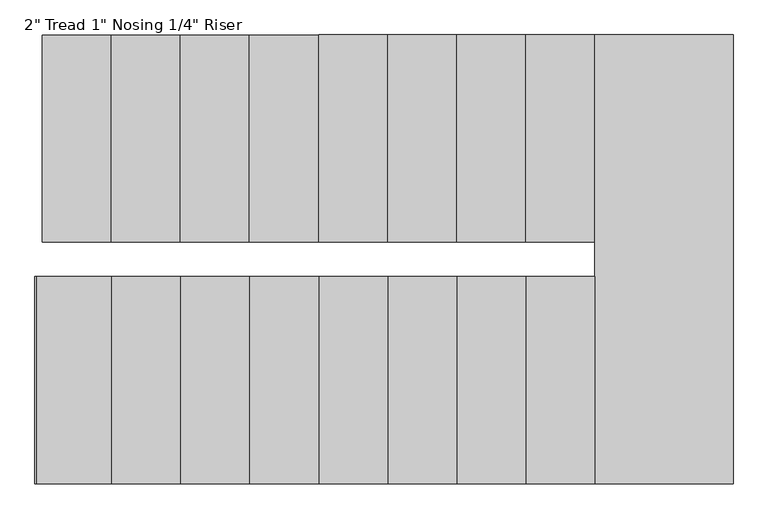
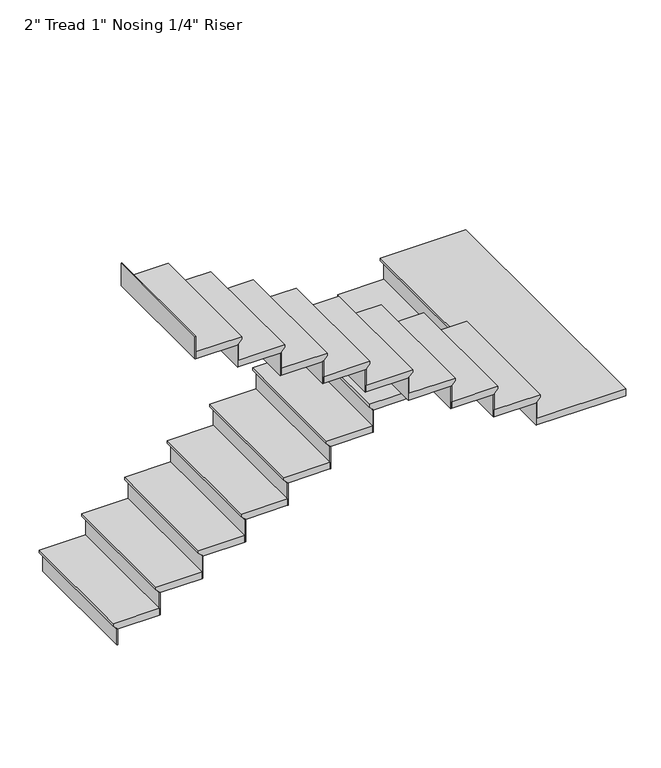
"""IFC4 building model written with IfcOpenShell, lengths in millimetres: stair flight geometry."""

from ifc_helpers import new_model, si_unit, origin, place, context, project, spatial, faceted_brep, source, transform, mapped, element, save


def stair_flight_0b98486b(model_context):
    return source(origin(), model_context, "Body", "Brep", [
        faceted_brep([(4699.0, 4356.1, 3198.2833333), (4699.0, 4356.1, 3217.3333333), (4699.0, 5270.5, 3217.3333333), (4699.0, 5270.5, 3198.2833333), (4724.4, 4356.1, 3172.8833333), (4724.4, 5270.5, 3172.8833333), (5029.2, 4356.1, 3217.3333333), (5029.2, 5270.5, 3217.3333333), (4724.4, 5270.5, 3166.5333333), (5029.2, 5270.5, 3166.5333333), (5029.2, 4356.1, 3166.5333333), (4724.4, 4356.1, 3166.5333333)], [[[0, 1, 2, 3]], [[4, 0, 3, 5]], [[2, 1, 6, 7]], [[8, 9, 10, 11]], [[2, 7, 9, 8, 5, 3]], [[8, 11, 4, 5]], [[6, 1, 0, 4, 11, 10]], [[7, 6, 10, 9]]]),
        faceted_brep([(4724.4, 4356.1, 3166.5333333), (4724.4, 4356.1, 3048.0), (4730.75, 4356.1, 3048.0), (4730.75, 4356.1, 3166.5333333), (4724.4, 5270.5, 3166.5333333), (4730.75, 5270.5, 3166.5333333), (4730.75, 5270.5, 3048.0), (4724.4, 5270.5, 3048.0)], [[[0, 1, 2, 3]], [[4, 5, 6, 7]], [[1, 0, 4, 7]], [[2, 1, 7, 6]], [[3, 2, 6, 5]], [[0, 3, 5, 4]]]),
        faceted_brep([(5029.2, 4356.1, 3335.8666667), (5029.2, 4356.1, 3166.5333333), (5035.55, 4356.1, 3166.5333333), (5035.55, 4356.1, 3335.8666667), (5029.2, 5270.5, 3335.8666667), (5035.55, 5270.5, 3335.8666667), (5035.55, 5270.5, 3166.5333333), (5029.2, 5270.5, 3166.5333333)], [[[0, 1, 2, 3]], [[4, 5, 6, 7]], [[1, 0, 4, 7]], [[2, 1, 7, 6]], [[3, 2, 6, 5]], [[0, 3, 5, 4]]]),
        faceted_brep([(5003.8, 5270.5, 3386.6666667), (5003.8, 4356.1, 3386.6666667), (5334.0, 4356.1, 3386.6666667), (5334.0, 5270.5, 3386.6666667), (5029.2, 5270.5, 3335.8666667), (5334.0, 5270.5, 3335.8666667), (5334.0, 4356.1, 3335.8666667), (5029.2, 4356.1, 3335.8666667), (5029.2, 5270.5, 3342.2166667), (5003.8, 5270.5, 3367.6166667), (5029.2, 4356.1, 3342.2166667), (5003.8, 4356.1, 3367.6166667)], [[[0, 1, 2, 3]], [[4, 5, 6, 7]], [[0, 3, 5, 4, 8, 9]], [[4, 7, 10, 8]], [[2, 1, 11, 10, 7, 6]], [[3, 2, 6, 5]], [[11, 1, 0, 9]], [[10, 11, 9, 8]]]),
        faceted_brep([(5334.0, 4356.1, 3505.2), (5334.0, 4356.1, 3335.8666667), (5340.35, 4356.1, 3335.8666667), (5340.35, 4356.1, 3505.2), (5334.0, 5270.5, 3505.2), (5340.35, 5270.5, 3505.2), (5340.35, 5270.5, 3335.8666667), (5334.0, 5270.5, 3335.8666667)], [[[0, 1, 2, 3]], [[4, 5, 6, 7]], [[1, 0, 4, 7]], [[2, 1, 7, 6]], [[3, 2, 6, 5]], [[0, 3, 5, 4]]]),
        faceted_brep([(5308.6, 5270.5, 3556.0), (5308.6, 4356.1, 3556.0), (5638.8, 4356.1, 3556.0), (5638.8, 5270.5, 3556.0), (5334.0, 5270.5, 3505.2), (5638.8, 5270.5, 3505.2), (5638.8, 4356.1, 3505.2), (5334.0, 4356.1, 3505.2), (5334.0, 5270.5, 3511.55), (5308.6, 5270.5, 3536.95), (5334.0, 4356.1, 3511.55), (5308.6, 4356.1, 3536.95)], [[[0, 1, 2, 3]], [[4, 5, 6, 7]], [[0, 3, 5, 4, 8, 9]], [[4, 7, 10, 8]], [[2, 1, 11, 10, 7, 6]], [[3, 2, 6, 5]], [[11, 1, 0, 9]], [[10, 11, 9, 8]]]),
        faceted_brep([(5638.8, 4356.1, 3674.5333333), (5638.8, 4356.1, 3505.2), (5645.15, 4356.1, 3505.2), (5645.15, 4356.1, 3674.5333333), (5638.8, 5270.5, 3674.5333333), (5645.15, 5270.5, 3674.5333333), (5645.15, 5270.5, 3505.2), (5638.8, 5270.5, 3505.2)], [[[0, 1, 2, 3]], [[4, 5, 6, 7]], [[1, 0, 4, 7]], [[2, 1, 7, 6]], [[3, 2, 6, 5]], [[0, 3, 5, 4]]]),
        faceted_brep([(5613.4, 5270.5, 3725.3333333), (5613.4, 4356.1, 3725.3333333), (5943.6, 4356.1, 3725.3333333), (5943.6, 5270.5, 3725.3333333), (5638.8, 5270.5, 3674.5333333), (5943.6, 5270.5, 3674.5333333), (5943.6, 4356.1, 3674.5333333), (5638.8, 4356.1, 3674.5333333), (5638.8, 5270.5, 3680.8833333), (5613.4, 5270.5, 3706.2833333), (5638.8, 4356.1, 3680.8833333), (5613.4, 4356.1, 3706.2833333)], [[[0, 1, 2, 3]], [[4, 5, 6, 7]], [[0, 3, 5, 4, 8, 9]], [[4, 7, 10, 8]], [[2, 1, 11, 10, 7, 6]], [[3, 2, 6, 5]], [[11, 1, 0, 9]], [[10, 11, 9, 8]]]),
        faceted_brep([(5943.6, 4356.1, 3843.8666667), (5943.6, 4356.1, 3674.5333333), (5949.95, 4356.1, 3674.5333333), (5949.95, 4356.1, 3843.8666667), (5943.6, 5270.5, 3843.8666667), (5949.95, 5270.5, 3843.8666667), (5949.95, 5270.5, 3674.5333333), (5943.6, 5270.5, 3674.5333333)], [[[0, 1, 2, 3]], [[4, 5, 6, 7]], [[1, 0, 4, 7]], [[2, 1, 7, 6]], [[3, 2, 6, 5]], [[0, 3, 5, 4]]]),
        faceted_brep([(5918.2, 5270.5, 3894.6666667), (5918.2, 4356.1, 3894.6666667), (6248.4, 4356.1, 3894.6666667), (6248.4, 5270.5, 3894.6666667), (5943.6, 5270.5, 3843.8666667), (6248.4, 5270.5, 3843.8666667), (6248.4, 4356.1, 3843.8666667), (5943.6, 4356.1, 3843.8666667), (5943.6, 5270.5, 3850.2166667), (5918.2, 5270.5, 3875.6166667), (5943.6, 4356.1, 3850.2166667), (5918.2, 4356.1, 3875.6166667)], [[[0, 1, 2, 3]], [[4, 5, 6, 7]], [[0, 3, 5, 4, 8, 9]], [[4, 7, 10, 8]], [[2, 1, 11, 10, 7, 6]], [[3, 2, 6, 5]], [[11, 1, 0, 9]], [[10, 11, 9, 8]]]),
        faceted_brep([(6248.4, 4356.1, 4013.2), (6248.4, 4356.1, 3843.8666667), (6254.75, 4356.1, 3843.8666667), (6254.75, 4356.1, 4013.2), (6248.4, 5270.5, 4013.2), (6254.75, 5270.5, 4013.2), (6254.75, 5270.5, 3843.8666667), (6248.4, 5270.5, 3843.8666667)], [[[0, 1, 2, 3]], [[4, 5, 6, 7]], [[1, 0, 4, 7]], [[2, 1, 7, 6]], [[3, 2, 6, 5]], [[0, 3, 5, 4]]]),
        faceted_brep([(6223.0, 5270.5, 4064.0), (6223.0, 4356.1, 4064.0), (6553.2, 4356.1, 4064.0), (6553.2, 5270.5, 4064.0), (6248.4, 5270.5, 4013.2), (6553.2, 5270.5, 4013.2), (6553.2, 4356.1, 4013.2), (6248.4, 4356.1, 4013.2), (6248.4, 5270.5, 4019.55), (6223.0, 5270.5, 4044.95), (6248.4, 4356.1, 4019.55), (6223.0, 4356.1, 4044.95)], [[[0, 1, 2, 3]], [[4, 5, 6, 7]], [[0, 3, 5, 4, 8, 9]], [[4, 7, 10, 8]], [[2, 1, 11, 10, 7, 6]], [[3, 2, 6, 5]], [[11, 1, 0, 9]], [[10, 11, 9, 8]]]),
        faceted_brep([(6553.2, 4356.1, 4182.5333333), (6553.2, 4356.1, 4013.2), (6559.55, 4356.1, 4013.2), (6559.55, 4356.1, 4182.5333333), (6553.2, 5270.5, 4182.5333333), (6559.55, 5270.5, 4182.5333333), (6559.55, 5270.5, 4013.2), (6553.2, 5270.5, 4013.2)], [[[0, 1, 2, 3]], [[4, 5, 6, 7]], [[1, 0, 4, 7]], [[2, 1, 7, 6]], [[3, 2, 6, 5]], [[0, 3, 5, 4]]]),
        faceted_brep([(6527.8, 5270.5, 4233.3333333), (6527.8, 4356.1, 4233.3333333), (6858.0, 4356.1, 4233.3333333), (6858.0, 5270.5, 4233.3333333), (6553.2, 5270.5, 4182.5333333), (6858.0, 5270.5, 4182.5333333), (6858.0, 4356.1, 4182.5333333), (6553.2, 4356.1, 4182.5333333), (6553.2, 5270.5, 4188.8833333), (6527.8, 5270.5, 4214.2833333), (6553.2, 4356.1, 4188.8833333), (6527.8, 4356.1, 4214.2833333)], [[[0, 1, 2, 3]], [[4, 5, 6, 7]], [[0, 3, 5, 4, 8, 9]], [[4, 7, 10, 8]], [[2, 1, 11, 10, 7, 6]], [[3, 2, 6, 5]], [[11, 1, 0, 9]], [[10, 11, 9, 8]]]),
        faceted_brep([(6858.0, 4356.1, 4351.8666667), (6858.0, 4356.1, 4182.5333333), (6864.35, 4356.1, 4182.5333333), (6864.35, 4356.1, 4351.8666667), (6858.0, 5270.5, 4351.8666667), (6864.35, 5270.5, 4351.8666667), (6864.35, 5270.5, 4182.5333333), (6858.0, 5270.5, 4182.5333333)], [[[0, 1, 2, 3]], [[4, 5, 6, 7]], [[1, 0, 4, 7]], [[2, 1, 7, 6]], [[3, 2, 6, 5]], [[0, 3, 5, 4]]]),
        faceted_brep([(6832.6, 5270.5, 4402.6666667), (6832.6, 4356.1, 4402.6666667), (7162.8, 4356.1, 4402.6666667), (7162.8, 5270.5, 4402.6666667), (6858.0, 5270.5, 4351.8666667), (7162.8, 5270.5, 4351.8666667), (7162.8, 4356.1, 4351.8666667), (6858.0, 4356.1, 4351.8666667), (6858.0, 5270.5, 4358.2166667), (6832.6, 5270.5, 4383.6166667), (6858.0, 4356.1, 4358.2166667), (6832.6, 4356.1, 4383.6166667)], [[[0, 1, 2, 3]], [[4, 5, 6, 7]], [[0, 3, 5, 4, 8, 9]], [[4, 7, 10, 8]], [[2, 1, 11, 10, 7, 6]], [[3, 2, 6, 5]], [[11, 1, 0, 9]], [[10, 11, 9, 8]]]),
        faceted_brep([(7162.8, 4356.1, 4521.2), (7162.8, 4356.1, 4351.8666667), (7169.15, 4356.1, 4351.8666667), (7169.15, 4356.1, 4521.2), (7162.8, 5270.5, 4521.2), (7169.15, 5270.5, 4521.2), (7169.15, 5270.5, 4351.8666667), (7162.8, 5270.5, 4351.8666667)], [[[0, 1, 2, 3]], [[4, 5, 6, 7]], [[1, 0, 4, 7]], [[2, 1, 7, 6]], [[3, 2, 6, 5]], [[0, 3, 5, 4]]]),
        faceted_brep([(7112.0, 3289.3, 4572.0), (7747.0, 3289.3, 4572.0), (7747.0, 5270.5, 4572.0), (7137.4, 5270.5, 4572.0), (7137.4, 4203.7, 4572.0), (7112.0, 4203.7, 4572.0), (7747.0, 3289.3, 4521.2), (7112.0, 3289.3, 4521.2), (7112.0, 4203.7, 4521.2), (7137.4, 4203.7, 4521.2), (7137.4, 4356.1, 4521.2), (7162.8, 4356.1, 4521.2), (7162.8, 5270.5, 4521.2), (7747.0, 5270.5, 4521.2), (7162.8, 5270.5, 4527.55), (7137.4, 5270.5, 4552.95), (7162.8, 4356.1, 4527.55), (7137.4, 4356.1, 4552.95)], [[[0, 1, 2, 3, 4, 5]], [[6, 7, 8, 9, 10, 11, 12, 13]], [[1, 0, 7, 6]], [[2, 1, 6, 13]], [[3, 2, 13, 12, 14, 15]], [[12, 11, 16, 14]], [[11, 10, 17, 16]], [[4, 3, 15, 17, 10, 9]], [[5, 4, 9, 8]], [[0, 5, 8, 7]], [[15, 14, 16, 17]]]),
        faceted_brep([(7112.0, 4203.7, 4690.5333333), (7112.0, 4203.7, 4521.2), (7105.65, 4203.7, 4521.2), (7105.65, 4203.7, 4690.5333333), (7112.0, 3289.3, 4690.5333333), (7105.65, 3289.3, 4690.5333333), (7105.65, 3289.3, 4521.2), (7112.0, 3289.3, 4521.2)], [[[0, 1, 2, 3]], [[4, 5, 6, 7]], [[1, 0, 4, 7]], [[2, 1, 7, 6]], [[3, 2, 6, 5]], [[0, 3, 5, 4]]]),
        faceted_brep([(7137.4, 3289.3, 4741.3333333), (7137.4, 4203.7, 4741.3333333), (6807.2, 4203.7, 4741.3333333), (6807.2, 3289.3, 4741.3333333), (7112.0, 3289.3, 4690.5333333), (6807.2, 3289.3, 4690.5333333), (6807.2, 4203.7, 4690.5333333), (7112.0, 4203.7, 4690.5333333), (7112.0, 3289.3, 4696.8833333), (7137.4, 3289.3, 4722.2833333), (7112.0, 4203.7, 4696.8833333), (7137.4, 4203.7, 4722.2833333)], [[[0, 1, 2, 3]], [[4, 5, 6, 7]], [[0, 3, 5, 4, 8, 9]], [[4, 7, 10, 8]], [[2, 1, 11, 10, 7, 6]], [[3, 2, 6, 5]], [[11, 1, 0, 9]], [[10, 11, 9, 8]]]),
        faceted_brep([(6807.2, 4203.7, 4859.8666667), (6807.2, 4203.7, 4690.5333333), (6800.85, 4203.7, 4690.5333333), (6800.85, 4203.7, 4859.8666667), (6807.2, 3289.3, 4859.8666667), (6800.85, 3289.3, 4859.8666667), (6800.85, 3289.3, 4690.5333333), (6807.2, 3289.3, 4690.5333333)], [[[0, 1, 2, 3]], [[4, 5, 6, 7]], [[1, 0, 4, 7]], [[2, 1, 7, 6]], [[3, 2, 6, 5]], [[0, 3, 5, 4]]]),
        faceted_brep([(6832.6, 3289.3, 4910.6666667), (6832.6, 4203.7, 4910.6666667), (6502.4, 4203.7, 4910.6666667), (6502.4, 3289.3, 4910.6666667), (6807.2, 3289.3, 4859.8666667), (6502.4, 3289.3, 4859.8666667), (6502.4, 4203.7, 4859.8666667), (6807.2, 4203.7, 4859.8666667), (6807.2, 3289.3, 4866.2166667), (6832.6, 3289.3, 4891.6166667), (6807.2, 4203.7, 4866.2166667), (6832.6, 4203.7, 4891.6166667)], [[[0, 1, 2, 3]], [[4, 5, 6, 7]], [[0, 3, 5, 4, 8, 9]], [[4, 7, 10, 8]], [[2, 1, 11, 10, 7, 6]], [[3, 2, 6, 5]], [[11, 1, 0, 9]], [[10, 11, 9, 8]]]),
        faceted_brep([(6502.4, 4203.7, 5029.2), (6502.4, 4203.7, 4859.8666667), (6496.05, 4203.7, 4859.8666667), (6496.05, 4203.7, 5029.2), (6502.4, 3289.3, 5029.2), (6496.05, 3289.3, 5029.2), (6496.05, 3289.3, 4859.8666667), (6502.4, 3289.3, 4859.8666667)], [[[0, 1, 2, 3]], [[4, 5, 6, 7]], [[1, 0, 4, 7]], [[2, 1, 7, 6]], [[3, 2, 6, 5]], [[0, 3, 5, 4]]]),
        faceted_brep([(6527.8, 3289.3, 5080.0), (6527.8, 4203.7, 5080.0), (6197.6, 4203.7, 5080.0), (6197.6, 3289.3, 5080.0), (6502.4, 3289.3, 5029.2), (6197.6, 3289.3, 5029.2), (6197.6, 4203.7, 5029.2), (6502.4, 4203.7, 5029.2), (6502.4, 3289.3, 5035.55), (6527.8, 3289.3, 5060.95), (6502.4, 4203.7, 5035.55), (6527.8, 4203.7, 5060.95)], [[[0, 1, 2, 3]], [[4, 5, 6, 7]], [[0, 3, 5, 4, 8, 9]], [[4, 7, 10, 8]], [[2, 1, 11, 10, 7, 6]], [[3, 2, 6, 5]], [[11, 1, 0, 9]], [[10, 11, 9, 8]]]),
        faceted_brep([(6197.6, 4203.7, 5198.5333333), (6197.6, 4203.7, 5029.2), (6191.25, 4203.7, 5029.2), (6191.25, 4203.7, 5198.5333333), (6197.6, 3289.3, 5198.5333333), (6191.25, 3289.3, 5198.5333333), (6191.25, 3289.3, 5029.2), (6197.6, 3289.3, 5029.2)], [[[0, 1, 2, 3]], [[4, 5, 6, 7]], [[1, 0, 4, 7]], [[2, 1, 7, 6]], [[3, 2, 6, 5]], [[0, 3, 5, 4]]]),
        faceted_brep([(6223.0, 3289.3, 5249.3333333), (6223.0, 4203.7, 5249.3333333), (5892.8, 4203.7, 5249.3333333), (5892.8, 3289.3, 5249.3333333), (6197.6, 3289.3, 5198.5333333), (5892.8, 3289.3, 5198.5333333), (5892.8, 4203.7, 5198.5333333), (6197.6, 4203.7, 5198.5333333), (6197.6, 3289.3, 5204.8833333), (6223.0, 3289.3, 5230.2833333), (6197.6, 4203.7, 5204.8833333), (6223.0, 4203.7, 5230.2833333)], [[[0, 1, 2, 3]], [[4, 5, 6, 7]], [[0, 3, 5, 4, 8, 9]], [[4, 7, 10, 8]], [[2, 1, 11, 10, 7, 6]], [[3, 2, 6, 5]], [[11, 1, 0, 9]], [[10, 11, 9, 8]]]),
        faceted_brep([(5892.8, 4203.7, 5367.8666667), (5892.8, 4203.7, 5198.5333333), (5886.45, 4203.7, 5198.5333333), (5886.45, 4203.7, 5367.8666667), (5892.8, 3289.3, 5367.8666667), (5886.45, 3289.3, 5367.8666667), (5886.45, 3289.3, 5198.5333333), (5892.8, 3289.3, 5198.5333333)], [[[0, 1, 2, 3]], [[4, 5, 6, 7]], [[1, 0, 4, 7]], [[2, 1, 7, 6]], [[3, 2, 6, 5]], [[0, 3, 5, 4]]]),
        faceted_brep([(5918.2, 3289.3, 5418.6666667), (5918.2, 4203.7, 5418.6666667), (5588.0, 4203.7, 5418.6666667), (5588.0, 3289.3, 5418.6666667), (5892.8, 3289.3, 5367.8666667), (5588.0, 3289.3, 5367.8666667), (5588.0, 4203.7, 5367.8666667), (5892.8, 4203.7, 5367.8666667), (5892.8, 3289.3, 5374.2166667), (5918.2, 3289.3, 5399.6166667), (5892.8, 4203.7, 5374.2166667), (5918.2, 4203.7, 5399.6166667)], [[[0, 1, 2, 3]], [[4, 5, 6, 7]], [[0, 3, 5, 4, 8, 9]], [[4, 7, 10, 8]], [[2, 1, 11, 10, 7, 6]], [[3, 2, 6, 5]], [[11, 1, 0, 9]], [[10, 11, 9, 8]]]),
        faceted_brep([(5588.0, 4203.7, 5537.2), (5588.0, 4203.7, 5367.8666667), (5581.65, 4203.7, 5367.8666667), (5581.65, 4203.7, 5537.2), (5588.0, 3289.3, 5537.2), (5581.65, 3289.3, 5537.2), (5581.65, 3289.3, 5367.8666667), (5588.0, 3289.3, 5367.8666667)], [[[0, 1, 2, 3]], [[4, 5, 6, 7]], [[1, 0, 4, 7]], [[2, 1, 7, 6]], [[3, 2, 6, 5]], [[0, 3, 5, 4]]]),
        faceted_brep([(5613.4, 3289.3, 5588.0), (5613.4, 4203.7, 5588.0), (5283.2, 4203.7, 5588.0), (5283.2, 3289.3, 5588.0), (5588.0, 3289.3, 5537.2), (5283.2, 3289.3, 5537.2), (5283.2, 4203.7, 5537.2), (5588.0, 4203.7, 5537.2), (5588.0, 3289.3, 5543.55), (5613.4, 3289.3, 5568.95), (5588.0, 4203.7, 5543.55), (5613.4, 4203.7, 5568.95)], [[[0, 1, 2, 3]], [[4, 5, 6, 7]], [[0, 3, 5, 4, 8, 9]], [[4, 7, 10, 8]], [[2, 1, 11, 10, 7, 6]], [[3, 2, 6, 5]], [[11, 1, 0, 9]], [[10, 11, 9, 8]]]),
        faceted_brep([(5283.2, 4203.7, 5706.5333333), (5283.2, 4203.7, 5537.2), (5276.85, 4203.7, 5537.2), (5276.85, 4203.7, 5706.5333333), (5283.2, 3289.3, 5706.5333333), (5276.85, 3289.3, 5706.5333333), (5276.85, 3289.3, 5537.2), (5283.2, 3289.3, 5537.2)], [[[0, 1, 2, 3]], [[4, 5, 6, 7]], [[1, 0, 4, 7]], [[2, 1, 7, 6]], [[3, 2, 6, 5]], [[0, 3, 5, 4]]]),
        faceted_brep([(5308.6, 3289.3, 5757.3333333), (5308.6, 4203.7, 5757.3333333), (4978.4, 4203.7, 5757.3333333), (4978.4, 3289.3, 5757.3333333), (5283.2, 3289.3, 5706.5333333), (4978.4, 3289.3, 5706.5333333), (4978.4, 4203.7, 5706.5333333), (5283.2, 4203.7, 5706.5333333), (5283.2, 3289.3, 5712.8833333), (5308.6, 3289.3, 5738.2833333), (5283.2, 4203.7, 5712.8833333), (5308.6, 4203.7, 5738.2833333)], [[[0, 1, 2, 3]], [[4, 5, 6, 7]], [[0, 3, 5, 4, 8, 9]], [[4, 7, 10, 8]], [[2, 1, 11, 10, 7, 6]], [[3, 2, 6, 5]], [[11, 1, 0, 9]], [[10, 11, 9, 8]]]),
        faceted_brep([(4978.4, 4203.7, 5875.8666667), (4978.4, 4203.7, 5706.5333333), (4972.05, 4203.7, 5706.5333333), (4972.05, 4203.7, 5875.8666667), (4978.4, 3289.3, 5875.8666667), (4972.05, 3289.3, 5875.8666667), (4972.05, 3289.3, 5706.5333333), (4978.4, 3289.3, 5706.5333333)], [[[0, 1, 2, 3]], [[4, 5, 6, 7]], [[1, 0, 4, 7]], [[2, 1, 7, 6]], [[3, 2, 6, 5]], [[0, 3, 5, 4]]]),
        faceted_brep([(4673.6, 4203.7, 6045.2), (4673.6, 4203.7, 5875.8666667), (4667.25, 4203.7, 5875.8666667), (4667.25, 4203.7, 6045.2), (4673.6, 3289.3, 6045.2), (4667.25, 3289.3, 6045.2), (4667.25, 3289.3, 5875.8666667), (4673.6, 3289.3, 5875.8666667)], [[[0, 1, 2, 3]], [[4, 5, 6, 7]], [[1, 0, 4, 7]], [[2, 1, 7, 6]], [[3, 2, 6, 5]], [[0, 3, 5, 4]]]),
        faceted_brep([(5003.8, 3289.3, 5926.6666667), (5003.8, 4203.7, 5926.6666667), (4673.6, 4203.7, 5926.6666667), (4673.6, 3289.3, 5926.6666667), (4978.4, 3289.3, 5875.8666667), (4673.6, 3289.3, 5875.8666667), (4673.6, 4203.7, 5875.8666667), (4978.4, 4203.7, 5875.8666667), (4978.4, 3289.3, 5882.2166667), (5003.8, 3289.3, 5907.6166667), (4978.4, 4203.7, 5882.2166667), (5003.8, 4203.7, 5907.6166667)], [[[0, 1, 2, 3]], [[4, 5, 6, 7]], [[0, 3, 5, 4, 8, 9]], [[4, 7, 10, 8]], [[2, 1, 11, 10, 7, 6]], [[3, 2, 6, 5]], [[11, 1, 0, 9]], [[10, 11, 9, 8]]]),
    ])


if __name__ == "__main__":
    model = new_model("IFC4")
    model_context = context("Model", 3, world=origin())
    ifc_project = project(units=[si_unit("LENGTHUNIT", "METRE", prefix="MILLI")], contexts=[model_context])
    site = spatial("IfcSite", under=ifc_project)
    building = spatial("IfcBuilding", under=site)
    placement = place(None, origin())
    stair_flight_shape = stair_flight_0b98486b(model_context)
    element("IfcStairFlight", 1, ObjectType="2\" Tread 1\" Nosing 1/4\" Riser", at=placement, inside=building, context=model_context, shape_type="MappedRepresentation", body=[
        mapped(stair_flight_shape, transform((0.0, 0.0, 0.0), x_axis=(1.0, 0.0, 0.0), y_axis=(0.0, 1.0, 0.0), z_axis=(0.0, 0.0, 1.0))),
    ])
    save(model, "model.ifc")
